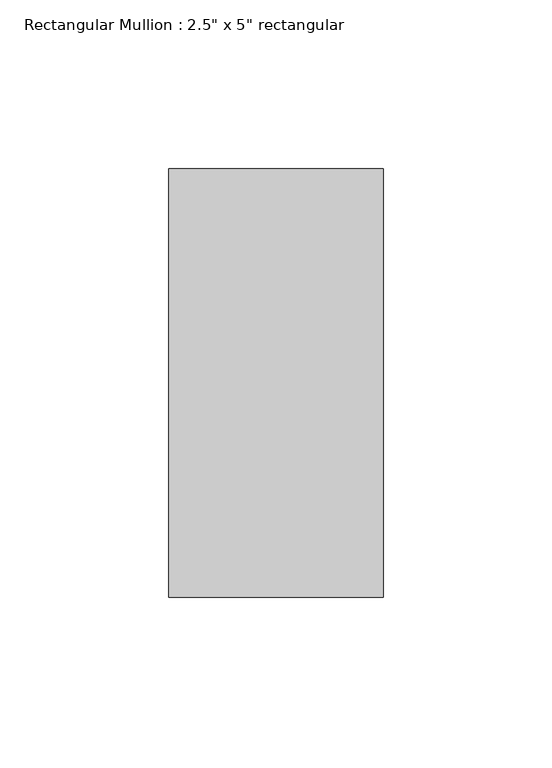
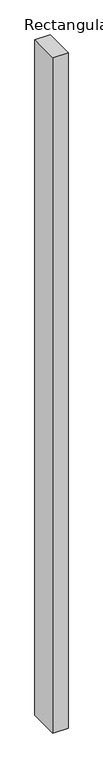
"""IFC4 building model written with IfcOpenShell, lengths in millimetres: member geometry."""

from ifc_helpers import new_model, si_unit, frame, origin, place, context, project, spatial, polyline, outline, extrude, source, transform, mapped, element, save


def member_71c27fd2(model_context):
    return source(origin(), model_context, "Body", "SweptSolid", [
        extrude(outline(polyline([(0.0, 63.5), (0.0, -63.5), (-63.5, -63.5), (-63.5, 63.5), (0.0, 63.5)])), frame((0.0, 0.0, -2952.7499997), z_axis=(0.0, 0.0, 1.0), x_axis=(1.0, 0.0, 0.0)), (0.0, 0.0, 1.0), 2952.7499997),
    ])


if __name__ == "__main__":
    model = new_model("IFC4")
    model_context = context("Model", 3, world=origin())
    ifc_project = project(units=[si_unit("LENGTHUNIT", "METRE", prefix="MILLI")], contexts=[model_context])
    site = spatial("IfcSite", under=ifc_project)
    building = spatial("IfcBuilding", under=site)
    placement = place(None, origin())
    member_shape = member_71c27fd2(model_context)
    element("IfcMember", 1, ObjectType="Rectangular Mullion : 2.5\" x 5\" rectangular", at=placement, inside=building, context=model_context, shape_type="MappedRepresentation", body=[
        mapped(member_shape, transform((0.0, 0.0, 0.0), x_axis=(1.0, 0.0, 0.0), y_axis=(0.0, 1.0, 0.0), z_axis=(0.0, 0.0, 1.0))),
    ])
    save(model, "model.ifc")

# Revit data of these elements
# Type "Rectangular Mullion : 2.5\" x 5\" rectangular"
#   built-in parameter 1007304 = 0.416667 (stored number, unit not read)
#   built-in parameter 1007301 = 0.104167 (stored number, unit not read)
#   built-in parameter 1007300 = 0.104167 (stored number, unit not read)
# Element 1 (IfcMember, "Rectangular Mullion : 2.5\" x 5\" rectangular")
#   Materials on its faces: "Aluminum"
# Materials
#   "Aluminum": class "Metal", colour RGB 247 247 247, transparency 0, Description = "Aluminum 6061", Cost = 0
